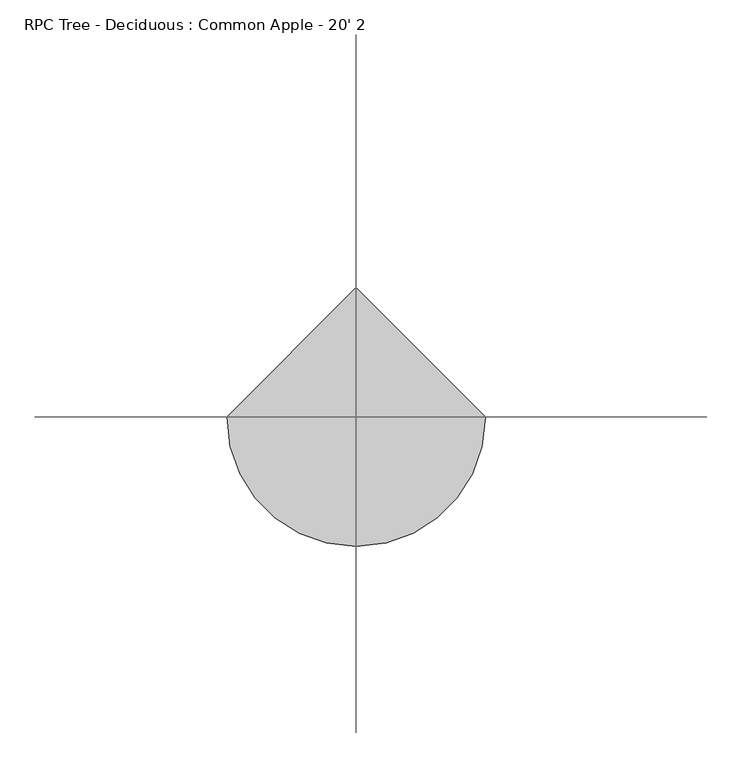
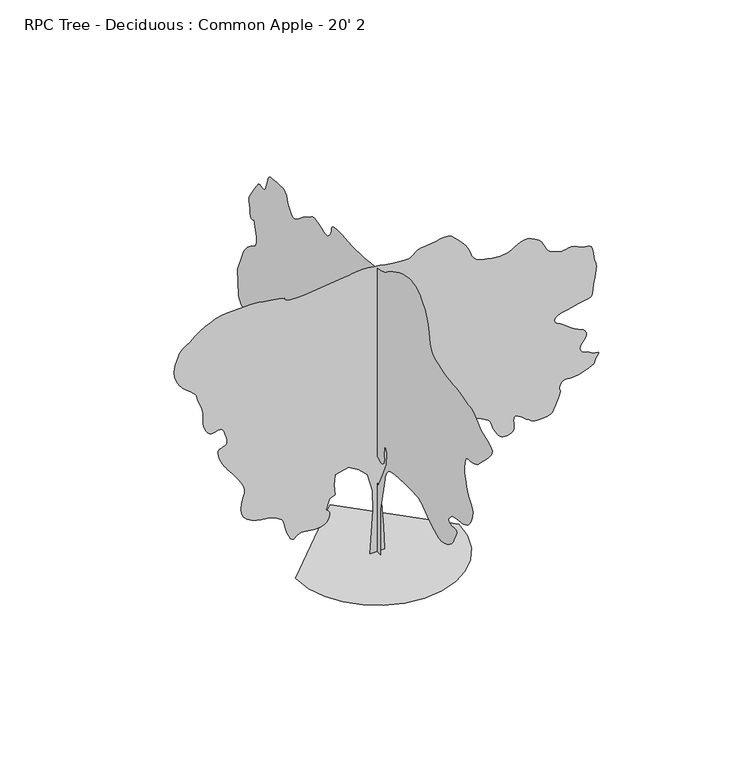
"""IFC4 building model written with IfcOpenShell, lengths in millimetres: geographic element geometry, RPC Tree - Deciduous : Common Apple - 20' 2."""

from ifc_helpers import new_model, si_unit, origin, place, context, project, spatial, triangles, source, transform, mapped, element, save


def rpc_tree_deciduous_common_apple_20_2_2cf08d23(model_context):
    return source(origin(), model_context, "Body", "Tessellation", [
        triangles([(-6.61e-05, -106.7031981, 0.0075972), (-6.25e-05, 141.1357166, 0.0075898), (-4.92e-05, 101.4814601, 465.9455781), (-3.19e-05, 131.2220957, 1031.0173004), (-1.83e-05, 230.3576144, 1437.4734501), (-8.7e-06, 398.8869896, 1675.3980263), (-1.1e-06, 587.2459139, 1834.016106), (2.7e-06, 765.6887283, 1873.6680462), (3.6e-06, 963.961219, 1804.2751888), (1.5e-06, 1023.4430534, 1705.1389435), (-4.1e-06, 904.4794573, 1576.2617809), (-8.5e-06, 944.1340136, 1407.7326782), (-1.46e-05, 1172.144878, 1090.4990622), (-1.49e-05, 1568.687534, 882.3128597), (-8.7e-06, 2143.6727863, 803.006436), (7.7e-06, 2490.6473923, 1179.7191977), (2.57e-05, 2847.5453751, 1606.0026981), (3.25e-05, 3402.6882339, 1556.4345028), (3.9e-05, 3600.9610153, 1675.3980263), (4.6e-05, 3591.0549339, 1913.3226025), (4.57e-05, 3412.6196045, 1992.6315697), (5.03e-05, 3283.7399712, 2210.7288677), (5.51e-05, 3591.0549339, 2220.6425068), (6.07e-05, 4205.6845688, 2101.6814541), (6.29e-05, 4275.3567696, 2137.8384041), (6.49e-05, 4342.3114037, 2174.2544952), (6.7e-05, 4403.9061905, 2211.1911942), (6.89e-05, 4457.4241447, 2248.9101128), (7.07e-05, 4500.1976967, 2287.6680668), (7.23e-05, 4529.5348595, 2327.7263775), (7.37e-05, 4542.7427742, 2369.3469475), (8.93e-05, 4572.4863075, 2874.9268433), (9.94e-05, 4403.9570595, 3301.215358), (0.0001002, 4386.5834106, 3334.8449913), (0.000101, 4360.9041641, 3374.6975006), (0.0001018, 4328.265168, 3418.5378479), (0.0001026, 4290.0887192, 3464.105706), (0.0001033, 4247.7471176, 3509.1651649), (0.0001039, 4202.636499, 3551.4561882), (0.0001043, 4156.1291634, 3588.718158), (0.0001045, 4111.323468, 3617.9027138), (0.0001046, 4070.8611122, 3640.1530998), (0.0001046, 4035.4281006, 3659.4571541), (0.0001048, 4005.7101471, 3679.8024239), (0.0001052, 3982.4182549, 3705.2026176), (0.000106, 3966.2384285, 3739.5941231), (0.0001073, 3957.8566727, 3786.9906487), (0.0001089, 3956.7898773, 3842.7945099), (0.0001107, 3961.4378494, 3899.6395866), (0.0001126, 3970.8614021, 3957.3738533), (0.0001145, 3984.0948967, 4015.7685448), (0.0001165, 4000.1982742, 4074.6966339), (0.0001185, 4018.2070587, 4133.9802246), (0.0001206, 4037.1553207, 4193.4417114), (0.0001203, 4062.5299347, 4172.9947037), (0.0001202, 4087.2188347, 4157.4244331), (0.0001204, 4110.5107269, 4151.5570587), (0.000121, 4131.7196068, 4160.2693176), (0.0001221, 4150.160051, 4188.3870781), (0.0001239, 4165.1460548, 4240.787368), (0.0001265, 4175.9410355, 4322.3213448), (0.000129, 4186.6092796, 4402.5600517), (0.0001308, 4198.1408432, 4455.5698975), (0.000132, 4205.3543564, 4492.9588943), (0.000133, 4202.9922913, 4526.3597626), (0.0001339, 4185.923275, 4567.406385), (0.0001352, 4148.8900703, 4627.7059021), (0.000137, 4086.736306, 4718.8666168), (0.0001389, 4019.8834099, 4816.9867905), (0.0001404, 3969.4896835, 4892.043837), (0.0001414, 3931.4405525, 4946.4759796), (0.0001421, 3901.5194138, 4982.6714447), (0.0001423, 3875.5858223, 5003.1184525), (0.0001421, 3849.5002052, 5010.2046478), (0.0001416, 3819.0709579, 5006.343837), (0.0001408, 3787.3208611, 4996.7176804), (0.0001401, 3759.4062859, 4987.6240494), (0.0001396, 3734.2601463, 4983.2045517), (0.0001394, 3710.841227, 4987.6240494), (0.0001396, 3688.1338921, 5005.0485672), (0.0001402, 3665.0704742, 5039.6435486), (0.0001416, 3640.6103394, 5095.574437), (0.0001432, 3619.2235634, 5160.9030075), (0.0001447, 3603.043737, 5219.9581238), (0.000146, 3587.5496246, 5271.4183548), (0.000147, 3568.2455704, 5313.8366959), (0.0001475, 3540.6103386, 5345.8661362), (0.0001475, 3500.1482735, 5366.109668), (0.0001469, 3442.3378487, 5373.1458664), (0.0001459, 3372.4368828, 5376.2445145), (0.0001451, 3300.6055115, 5383.3312912), (0.0001442, 3229.8412262, 5391.1034912), (0.0001434, 3163.0391991, 5396.2851517), (0.0001425, 3103.1713417, 5395.5485687), (0.0001414, 3053.2095657, 5385.642778), (0.0001402, 3016.0746231, 5363.2394943), (0.0001391, 2991.8429626, 5337.2044556), (0.0001382, 2976.4758774, 5316.3510773), (0.0001375, 2966.6462448, 5297.4283951), (0.0001368, 2959.0769394, 5277.1081238), (0.0001359, 2950.4664185, 5252.1148819), (0.0001348, 2937.5122673, 5219.1198029), (0.0001331, 2916.9382324, 5174.873085), (0.0001313, 2890.1666107, 5126.1051315), (0.0001296, 2860.6265533, 5083.2042618), (0.000128, 2827.9619774, 5048.4569641), (0.0001268, 2791.8432518, 5024.124147), (0.0001258, 2751.8890045, 5012.4399765), (0.0001253, 2707.794603, 5015.6909409), (0.0001252, 2659.1789658, 5036.0873703), (0.0001254, 2610.791803, 5068.0662323), (0.0001258, 2565.8846603, 5103.6768494), (0.0001263, 2521.8332794, 5141.7006912), (0.0001267, 2476.0523529, 5180.9436447), (0.0001272, 2425.9356445, 5220.212178), (0.0001274, 2368.8821503, 5258.2360199), (0.0001275, 2302.2908661, 5293.846637), (0.0001276, 2240.2945049, 5328.4671982), (0.0001279, 2193.5584042, 5362.0459625), (0.0001282, 2154.2798424, 5391.129071), (0.0001282, 2114.6558075, 5412.2365036), (0.0001278, 2066.8783459, 5421.8882401), (0.0001267, 2003.1496777, 5416.6304214), (0.0001247, 1915.6618492, 5392.9830276), (0.0001224, 1826.1497257, 5361.2837997), (0.0001207, 1757.9710384, 5335.9853439), (0.0001194, 1705.7434124, 5319.8816757), (0.0001187, 1664.0950825, 5315.7418121), (0.0001184, 1627.6484699, 5326.358606), (0.0001187, 1591.0293388, 5354.4766571), (0.0001195, 1548.8602558, 5402.8893997), (0.0001207, 1514.8419834, 5459.7853455), (0.000122, 1498.8602554, 5510.7630478), (0.0001232, 1489.8128426, 5554.806871), (0.0001241, 1476.6047825, 5590.874437), (0.0001244, 1448.1338459, 5617.9256927), (0.0001241, 1393.3079773, 5634.9182602), (0.0001229, 1301.0220406, 5640.8109238), (0.0001214, 1201.3955635, 5639.6935501), (0.0001202, 1126.7398006, 5636.6454803), (0.0001192, 1069.2519579, 5632.2259827), (0.0001184, 1021.1290958, 5626.9425842), (0.0001175, 974.5682751, 5621.3039749), (0.0001165, 921.7642307, 5615.8426804), (0.0001154, 854.9113346, 5611.0679718), (0.0001143, 784.7082069, 5608.019902), (0.0001133, 723.0014357, 5607.2071609), (0.0001125, 663.7228592, 5608.4768509), (0.0001116, 600.8019178, 5611.6516571), (0.0001107, 528.1680156, 5616.5792633), (0.0001096, 439.7556433, 5623.0567749), (0.0001082, 329.4941322, 5630.9051331), (0.0001067, 206.9466705, 5641.7254028), (0.0001053, 88.3885184, 5656.6861176), (0.0001042, -22.1921751, 5675.1262711), (0.0001034, -120.8075788, 5696.3354416), (0.0001029, -203.4686488, 5719.6276245), (0.0001027, -266.1871316, 5744.3162338), (0.0001028, -304.9729546, 5769.6908478), (0.0001032, -347.9523442, 5804.4381454), (0.0001036, -420.583703, 5853.4089935), (0.0001039, -514.8939712, 5910.1532043), (0.000104, -622.9024584, 5968.31884), (0.0001039, -736.6335978, 6021.4301331), (0.0001035, -848.1092062, 6063.1118912), (0.0001027, -949.3562239, 6086.9371811), (0.0001016, -1039.2697763, 6095.8017563), (0.0001004, -1122.4243664, 6096.0046509), (9.9e-05, -1199.3330441, 6086.1494385), (9.73e-05, -1270.5191059, 6064.8391113), (9.53e-05, -1336.5033051, 6030.7016602), (9.29e-05, -1397.8062492, 5982.3650757), (9.01e-05, -1454.9462208, 5918.407933), (8.77e-05, -1502.3755932, 5861.1056168), (8.62e-05, -1536.9730453, 5825.4944183), (8.5e-05, -1562.8963177, 5799.256485), (8.38e-05, -1584.313615, 5770.0716385), (8.22e-05, -1605.3828232, 5725.6220261), (7.96e-05, -1630.2698215, 5653.5874695), (7.58e-05, -1663.1323505, 5541.6751144), (7.16e-05, -1693.8258259, 5415.6147858), (6.81e-05, -1715.6747829, 5307.5626602), (6.5e-05, -1738.0446384, 5214.9799393), (6.21e-05, -1770.3000824, 5135.1981812), (5.93e-05, -1821.8062408, 5065.6530075), (5.62e-05, -1901.9230076, 5003.7532974), (5.28e-05, -2020.0178341, 4946.8823502), (4.95e-05, -2152.913356, 4902.7117905), (4.69e-05, -2273.494804, 4876.3974083), (4.48e-05, -2385.2295536, 4861.5384315), (4.29e-05, -2491.5921021, 4851.7340881), (4.1e-05, -2596.0345642, 4840.5071571), (3.89e-05, -2702.0542557, 4821.482737), (3.62e-05, -2813.1030006, 4788.2594742), (3.39e-05, -2912.3155495, 4758.5159409), (3.24e-05, -2986.585144, 4746.9843773), (3.14e-05, -3044.8780975, 4742.742485), (3.04e-05, -3096.2371719, 4734.8432579), (2.89e-05, -3149.6786774, 4712.3896866), (2.66e-05, -3214.2200867, 4664.4344742), (2.28e-05, -3298.878582, 4580.0809021), (1.85e-05, -3408.6320572, 4492.8062874), (1.5e-05, -3530.0185432, 4434.3354378), (1.2e-05, -3644.3188339, 4390.95233), (9.4e-06, -3732.7616913, 4348.9659393), (7.2e-06, -3776.6273277, 4294.6608238), (5.1e-06, -3757.196537, 4214.3459587), (3e-06, -3655.7486595, 4094.3056114), (1.1e-06, -3529.027906, 3968.7786804), (-3e-07, -3439.3912262, 3876.7287758), (-1.3e-06, -3376.6531952, 3811.5525215), (-1.9e-06, -3330.5522301, 3766.670668), (-2.3e-06, -3290.852037, 3735.479258), (-2.3e-06, -3247.3671913, 3711.4002045), (-2.2e-06, -3189.8108208, 3687.854258), (-1.7e-06, -3124.3802216, 3671.1919029), (-1e-06, -3064.487075, 3666.3404549), (-2e-07, -3010.8420937, 3664.4356293), (2e-07, -2964.1568619, 3656.6378494), (2e-07, -2925.0662247, 3634.0825401), (-8e-07, -2894.3070557, 3587.9559952), (-2.8e-06, -2872.5897766, 3509.3939301), (-5.1e-06, -2860.8041588, 3423.8465355), (-7.1e-06, -2858.3659355, 3357.9081184), (-8.8e-06, -2863.7507813, 3304.4410332), (-1.04e-05, -2875.358503, 3256.3335045), (-1.21e-05, -2891.6653564, 3206.498465), (-1.41e-05, -2911.070858, 3147.8244301), (-1.67e-05, -2932.0768433, 3073.199334), (-1.95e-05, -2961.2613991, 2993.8242371), (-2.22e-05, -3001.7234642, 2923.6186386), (-2.47e-05, -3046.5291595, 2859.6612053), (-2.72e-05, -3088.7187355, 2798.9806068), (-2.95e-05, -3121.3830208, 2738.6555099), (-3.16e-05, -3137.5628471, 2675.7398735), (-3.35e-05, -3130.349334, 2607.2612045), (-3.52e-05, -3109.3942177, 2540.281572), (-3.66e-05, -3087.7280983, 2482.819091), (-3.77e-05, -3063.4964378, 2433.5098915), (-3.85e-05, -3034.7182526, 2390.964814), (-3.91e-05, -2999.5645844, 2353.7970245), (-3.94e-05, -2956.0544495, 2320.6169277), (-3.96e-05, -2902.3333099, 2290.0378349), (-3.93e-05, -2836.3948929, 2266.2507694), (-3.86e-05, -2760.9314758, 2251.4832115), (-3.77e-05, -2680.9721123, 2241.3942924), (-3.68e-05, -2601.4955681, 2231.6559334), (-3.61e-05, -2527.6041481, 2217.9272655), (-3.58e-05, -2464.279525, 2195.8749779), (-3.62e-05, -2416.56049, 2161.1632885), (-3.68e-05, -2383.2356346, 2123.2410393), (-3.73e-05, -2359.9691769, 2093.2995529), (-3.79e-05, -2347.1065899, 2069.598674), (-3.84e-05, -2344.9984337, 2050.4090023), (-3.9e-05, -2353.9875652, 2033.9929985), (-3.98e-05, -2374.4217831, 2018.6158848), (-4.07e-05, -2406.646851, 2002.5452087), (-4.16e-05, -2449.8269188, 1993.9041664), (-4.23e-05, -2498.3841293, 1996.5330757), (-4.28e-05, -2545.5646797, 2002.2862129), (-4.34e-05, -2584.5791588, 2003.0075352), (-4.41e-05, -2608.6837921, 1990.5513187), (-4.52e-05, -2611.0967262, 1956.7642822), (-4.66e-05, -2585.0869766, 1893.4953243), (-4.83e-05, -2549.9080193, 1821.1814243), (-4.96e-05, -2524.6272949, 1762.91376), (-5.07e-05, -2502.1126808, 1714.5318295), (-5.16e-05, -2475.2625755, 1671.8725147), (-5.23e-05, -2436.9668026, 1630.7726978), (-5.27e-05, -2380.1140228, 1587.0720222), (-5.3e-05, -2297.5969666, 1536.6072247), (-5.28e-05, -2203.8378639, 1496.8968578), (-5.19e-05, -2116.842738, 1484.7582092), (-5.03e-05, -2034.8743401, 1494.9892708), (-4.83e-05, -1956.2028339, 1522.3883251), (-4.6e-05, -1879.090971, 1561.7532188), (-4.35e-05, -1801.803828, 1607.8822346), (-4.09e-05, -1722.6115688, 1655.5707481), (-3.83e-05, -1647.9584221, 1703.6352562), (-3.59e-05, -1583.013113, 1752.3931812), (-3.37e-05, -1524.1383636, 1798.8980461), (-3.16e-05, -1467.6919544, 1840.2010483), (-2.97e-05, -1410.0313751, 1873.3506237), (-2.82e-05, -1347.5167316, 1895.4053822), (-2.69e-05, -1276.503479, 1903.4089634), (-2.54e-05, -1177.6846561, 1904.2776604), (-2.33e-05, -1044.3574018, 1905.4916851), (-2.11e-05, -891.7820492, 1904.9710773), (-1.89e-05, -735.2163151, 1900.6352955), (-1.7e-05, -589.9230761, 1890.4040886), (-1.58e-05, -471.1627742, 1872.1948803), (-1.55e-05, -394.1956335, 1843.9297451), (-1.6e-05, -348.7041879, 1805.3140789), (-1.68e-05, -313.0958962, 1758.377409), (-1.8e-05, -285.7248199, 1704.5039532), (-1.95e-05, -264.9450744, 1645.0805454), (-2.11e-05, -249.1058704, 1581.494165), (-2.29e-05, -236.5620685, 1515.1341167), (-2.48e-05, -225.6659676, 1447.3870892), (-3.91e-05, -116.6168281, 912.0537769), (-2.05e-05, -27.3946828, 1318.5099266), (-1.32e-05, -176.0980811, 1635.74347), (-6.6e-06, -304.975498, 1923.2362415), (2e-07, -324.8002327, 2161.1632885), (4.8e-06, -255.4073572, 2280.1241959), (-4e-07, -225.6657133, 2091.767815), (-1.7e-06, -231.7353101, 2049.4539734), (-3e-06, -235.984215, 2008.1814926), (-4.2e-06, -236.5910275, 1968.9892628), (-5.2e-06, -231.7353101, 1932.9186447), (-6e-06, -219.5961346, 1901.0111446), (-6.5e-06, -198.3530817, 1874.3056526), (-6.6e-06, -166.1844602, 1853.8433842), (-6.2e-06, -129.2182845, 1848.5829494), (-5.3e-06, -95.0268123, 1860.3152275), (-4.3e-06, -63.9562343, 1879.3348515), (-3.4e-06, -36.354542, 1895.9235191), (-2.9e-06, -12.5678035, 1900.3761543), (-3.1e-06, 7.0569383, 1882.9772163), (-4.4e-06, 22.1729471, 1834.016106), (-6.1e-06, 32.8958209, 1768.9260384), (-7.8e-06, 39.9768386, 1709.0403042), (-9.4e-06, 44.0233167, 1653.4904972), (-1.1e-05, 45.6418044, 1601.4077751), (-1.24e-05, 45.4396183, 1551.9260571), (-1.39e-05, 44.0233167, 1504.1789715), (-1.53e-05, 41.9999482, 1457.3007282), (139.590126, 0.0003305, 0.0), (-135.4471285, 0.0003387, 0.0), (-74.3278259, 0.000241, 845.4879272), (-84.5142454, 0.0002472, 1242.76455), (-186.3807747, 0.0002013, 1599.294532), (-339.1791879, 0.0002082, 1752.0933449), (-542.9102117, 0.000216, 1874.3335579), (-797.5758808, 0.0002227, 1813.2134514), (-817.9492012, 0.0002203, 1609.4824276), (-797.5758808, 0.0002168, 1415.9368286), (-899.4426281, 0.0002191, 1365.0021469), (-970.7481594, 0.0002183, 1171.4565479), (-951.3247084, 0.0002718, 1158.1240768), (-933.2373676, 0.000271, 1143.3616058), (-917.8246456, 0.0002703, 1125.7517796), (-906.4200365, 0.0002696, 1103.8645981), (-900.3621214, 0.000269, 1076.2750757), (-900.9870106, 0.0002686, 1041.555756), (-909.6280529, 0.0002682, 998.2868128), (-928.5764603, 0.0002681, 955.1042742), (-957.6798437, 0.0002684, 921.0098436), (-994.6267164, 0.0002692, 895.1144766), (-1037.0955631, 0.0002701, 876.5217161), (-1082.7698101, 0.0002713, 864.3449158), (-1129.3382612, 0.0002726, 857.6926329), (-1174.4791832, 0.0002739, 855.6733521), (-1218.6700905, 0.0002753, 858.4063974), (-1263.5747623, 0.0002767, 865.0586803), (-1308.6573303, 0.0002782, 873.3161705), (-1353.3816353, 0.0002796, 880.857498), (-1397.217041, 0.000281, 885.3710306), (-1439.6273884, 0.0002823, 884.5404854), (-1480.0769543, 0.0002833, 876.0466724), (-1514.854628, 0.0002841, 857.900905), (-1542.5051205, 0.0002846, 834.4084436), (-1565.8782578, 0.000285, 812.6990856), (-1587.8238659, 0.0002854, 799.9000122), (-1611.1970032, 0.0002862, 803.1359339), (-1638.8473503, 0.0002874, 829.5392641), (-1673.6225533, 0.000235, 886.2346407), (-1706.6171963, 0.0002371, 959.4984827), (-1729.2790398, 0.0002388, 1029.5593225), (-1744.988982, 0.0002402, 1094.4487484), (-1757.1353336, 0.0002415, 1152.2135365), (-1769.1037891, 0.0002426, 1200.8900711), (-1784.2803337, 0.0002436, 1238.5177162), (-1806.0481911, 0.0002446, 1263.1378704), (-1833.1626698, 0.0002457, 1282.7670502), (-1863.3073414, 0.0002469, 1305.4288937), (-1898.2629112, 0.0002483, 1329.1576778), (-1939.8122646, 0.0002499, 1351.9948013), (-1989.7334908, 0.0002517, 1371.9820988), (-2049.8147072, 0.0002537, 1387.1586433), (-2121.8338577, 0.000256, 1395.5635082), (-2205.4938675, 0.0002044, 1404.6210949), (-2294.67854, 0.0002073, 1424.3695988), (-2382.4381542, 0.0002104, 1456.7724174), (-2461.8232796, 0.0002135, 1503.7853909), (-2525.8821602, 0.0002163, 1567.3691551), (-2567.6627495, 0.0002188, 1649.4849277), (-2580.2355286, 0.0002207, 1752.0933449), (-2568.9835991, 0.0002218, 1851.4048702), (-2548.8159348, 0.0002224, 1927.9097935), (-2527.0379036, 0.0002227, 1989.979842), (-2510.9723145, 0.0001688, 2045.9893593), (-2507.9117455, 0.0001695, 2104.3180664), (-2525.1659248, 0.0001711, 2173.3375454), (-2570.0503944, 0.0001737, 2261.4222851), (-2629.7912247, 0.0001769, 2355.7756828), (-2686.3316689, 0.0001798, 2438.7243988), (-2738.9604332, 0.0001825, 2511.3356644), (-2786.9665146, 0.0001849, 2574.6730774), (-2829.6130394, 0.0001327, 2629.841803), (-2866.1890045, 0.0001345, 2677.8478844), (-2896.008696, 0.000136, 2719.8086952), (-2924.6092758, 0.0001376, 2767.4084061), (-2955.1652596, 0.0001394, 2827.2762634), (-2983.4100471, 0.0001412, 2893.0114952), (-3005.0764572, 0.0001428, 2958.2389091), (-3015.8461487, 0.000144, 3016.5062828), (-3011.4772293, 0.0001446, 3061.4137161), (-2987.7028084, 0.0001442, 3086.5342758), (-2951.4823448, 0.0001433, 3098.8532913), (-2915.109565, 0.0001425, 3111.5533882), (-2882.1147766, 0.0001417, 3127.4282913), (-2856.0800285, 0.0001413, 3149.3740448), (-2840.5350471, 0.0001413, 3180.2349518), (-2839.0871704, 0.0001418, 3222.8561874), (-2855.2669968, 0.0001432, 3280.0823456), (-2877.0348541, 9.05e-05, 3338.9342766), (-2892.2240433, 9.16e-05, 3385.5177704), (-2904.1875572, 9.25e-05, 3421.2048363), (-2916.3286766, 9.32e-05, 3447.4686401), (-2932.0259743, 9.4e-05, 3465.705899), (-2954.70802, 9.48e-05, 3477.3389099), (-2987.7028084, 9.59e-05, 3483.8161308), (-3026.4123642, 9.7e-05, 3481.8857254), (-3064.2583099, 9.8e-05, 3472.1066711), (-3101.5455688, 9.9e-05, 3461.6419029), (-3138.6805115, 0.0001, 3457.552327), (-3175.9930595, 0.0001013, 3467.026458), (-3213.8137161, 0.0001029, 3497.1763618), (-3252.5488518, 0.0001049, 3555.1138138), (-3281.1747208, 0.0001068, 3626.7419998), (-3293.239682, 0.0001082, 3695.3474052), (-3295.8558014, 0.0001093, 3764.1307068), (-3296.1351448, 0.0001104, 3836.3175797), (-3301.2406471, 5.74e-05, 3915.0575409), (-3318.2840836, 5.93e-05, 4003.6274254), (-3354.4028091, 6.19e-05, 4105.2020393), (-3391.2836975, 6.43e-05, 4197.0231789), (-3411.2481766, 6.59e-05, 4259.8120789), (-3422.2972115, 6.68e-05, 4301.925206), (-3432.4570564, 6.76e-05, 4331.7448975), (-3449.7545471, 6.85e-05, 4357.6276199), (-3482.1650688, 6.99e-05, 4387.9804184), (-3537.7657448, 7.22e-05, 4431.1606316), (-3609.6985634, 2.09e-05, 4488.5646858), (-3681.631382, 2.41e-05, 4556.1285851), (-3747.3157448, 2.72e-05, 4634.0305161), (-3800.5287758, 3.01e-05, 4722.4480843), (-3835.047599, 3.26e-05, 4821.5588951), (-3844.6231773, 3.45e-05, 4931.5152649), (-3822.9823471, 3.57e-05, 5052.5468307), (-3789.555899, -1.8e-05, 5157.9310959), (-3763.7749146, -1.77e-05, 5228.187854), (-3739.5941231, -1.77e-05, 5274.3902664), (-3710.9682541, -1.81e-05, 5307.5882401), (-3671.8270386, -1.88e-05, 5338.8555176), (-3616.1246246, -1.98e-05, 5379.1652664), (-3537.7657448, -2.13e-05, 5439.6429703), (-3445.4364967, -2.3e-05, 5511.6775269), (-3351.6849518, -2.48e-05, 5578.225209), (-3256.3079247, -2.67e-05, 5637.4326416), (-3159.1783882, -2.89e-05, 5687.5726044), (-3060.0675774, -3.12e-05, 5726.8155579), (-2958.8228851, -3.39e-05, 5753.4348633), (-2855.2669968, -3.68e-05, 5765.6015625), (-2376.4970924, -5.09e-05, 5775.7869873), (-2309.7356152, -5.29e-05, 5773.1197083), (-2232.8167637, -5.53e-05, 5765.6521408), (-2147.4320045, -3.8e-06, 5754.1458664), (-2055.2781818, -6.7e-06, 5739.4392059), (-1958.0469074, -9.9e-06, 5722.3449005), (-1857.4273224, -1.32e-05, 5703.6251129), (-1755.1159801, -1.65e-05, 5684.1181641), (-1751.9080364, -1.69e-05, 5664.6617935), (-1742.5530842, -1.75e-05, 5646.3739563), (-1720.9022255, -1.83e-05, 5630.3970245), (-1680.8107773, -1.97e-05, 5617.9001129), (-1616.1270802, -2.18e-05, 5610.0261749), (-1520.7042709, -2.46e-05, 5607.9437439), (-1388.3981026, -2.85e-05, 5612.8201904), (-614.2181774, -5.02e-05, 5704.4890137), (-538.3076946, -5.24e-05, 5711.4996323), (-472.1990845, 1e-07, 5721.8879517), (-409.4762778, -1.6e-06, 5732.8355392), (-343.7232419, -3.5e-06, 5741.4460602), (-268.5264692, -5.7e-06, 5744.8749207), (-177.4707081, -8.5e-06, 5740.3031067), (-64.1414019, -1.21e-05, 5724.8598633), (54.7118994, -1.59e-05, 5704.3111176), (159.4882483, -1.93e-05, 5686.4296509), (252.3260954, -2.23e-05, 5671.4183578), (335.3640864, -2.49e-05, 5659.4039749), (410.7386644, -2.73e-05, 5650.6155579), (480.5886887, -2.95e-05, 5645.205423), (547.0529457, -3.15e-05, 5643.3764648), (603.2428662, -3.3e-05, 5651.8346695), (646.0698669, -3.4e-05, 5673.6531052), (683.3697704, -3.47e-05, 5703.4983765), (722.9887184, -3.54e-05, 5736.0359253), (772.7625698, -3.64e-05, 5765.8806152), (840.5349592, -3.81e-05, 5787.6996323), (934.1441437, -4.07e-05, 5796.1828354), (1035.6832947, -4.37e-05, 5802.989978), (1124.0372766, -4.61e-05, 5818.3826431), (1202.2337391, -4.82e-05, 5834.6642075), (1273.3004768, -5.01e-05, 5844.1636276), (1340.2726971, -5.22e-05, 5839.2360214), (1406.173035, -5.46e-05, 5812.2103455), (1474.0342999, -3.2e-06, 5755.4161377), (1539.0152172, -6.2e-06, 5686.9627579), (1594.7301304, -8.7e-06, 5628.1366974), (1641.8903332, -1.09e-05, 5576.0666199), (1681.2120609, -1.28e-05, 5527.9335114), (1713.4041367, -1.44e-05, 5480.8671982), (1739.182505, -1.59e-05, 5431.9975067), (1759.2587505, -1.73e-05, 5378.5304214), (1777.3156425, -1.87e-05, 5324.8604416), (1798.9361252, -2e-05, 5277.2604401), (1827.6839344, -2.15e-05, 5235.5281036), (1867.1225155, 3.1e-05, 5199.4855362), (1920.8180752, 2.9e-05, 5169.0060013), (1992.3318787, 2.65e-05, 5143.8342819), (2085.229842, 2.34e-05, 5123.844223), (2181.6306438, 2.03e-05, 5109.4171967), (2262.7075264, 1.78e-05, 5100.6799393), (2330.5991673, 1.57e-05, 5097.123761), (2387.4419186, 1.4e-05, 5098.1905563), (2435.3767834, 1.27e-05, 5103.3722168), (2476.5374977, 1.16e-05, 5112.0844757), (2513.0678261, 1.07e-05, 5123.844223), (2552.2195061, 9.8e-06, 5144.4947067), (2599.1840813, 8.9e-06, 5175.4829315), (2653.1336952, 7.8e-06, 5209.6459625), (2713.1032906, 6.4e-06, 5239.9226028), (2778.2795448, 4.8e-06, 5259.1249191), (2847.697982, 2.7e-06, 5260.1661346), (2920.5196999, 2e-07, 5235.9094757), (2984.2992371, -2.2e-06, 5202.1528152), (3030.2478859, -4e-06, 5176.5747253), (3062.9883293, -5.3e-06, 5154.908606), (3087.1947006, -6.3e-06, 5132.9122742), (3107.4893921, -7.3e-06, 5106.2679703), (3128.4697975, -8.5e-06, 5070.73293), (3154.8094688, -1e-05, 5021.9905563), (3182.8510712, 4.27e-05, 4971.0890121), (3208.2256851, 4.13e-05, 4930.3473129), (3234.4639091, 4e-05, 4897.4289734), (3265.1724998, 3.87e-05, 4870.0475052), (3303.9076355, 3.72e-05, 4845.8667137), (3354.2252037, 3.53e-05, 4822.6004013), (3419.6808014, 3.3e-05, 4797.8859215), (3486.0258797, 3.08e-05, 4782.8237595), (3540.0769409, 2.92e-05, 4784.7032959), (3586.9909378, 2.8e-05, 4795.4729874), (3631.9489494, 2.68e-05, 4807.1571579), (3680.1326363, 2.55e-05, 4811.7036827), (3736.6730804, 2.36e-05, 4801.0863075), (3806.7519424, 2.1e-05, 4767.3299377), (3879.2181587, 1.84e-05, 4732.9890106), (3939.9240463, 1.63e-05, 4718.4346664), (3989.5811897, 1.48e-05, 4712.2626595), (4028.9003014, 1.35e-05, 4703.0678719), (4058.6185455, 1.22e-05, 4679.4204781), (4079.3957657, 6.51e-05, 4629.9412308), (4091.9941246, 6.34e-05, 4543.2253029), (4103.8306114, 6.18e-05, 4454.6301292), (4119.4261711, 6.04e-05, 4397.0481789), (4135.0217308, 5.94e-05, 4355.3161331), (4146.8835068, 5.84e-05, 4314.2950905), (4151.2268463, 5.74e-05, 4258.8467308), (4144.3688347, 5.64e-05, 4173.8330246), (4122.550399, 5.51e-05, 4044.0642014), (4100.096537, 0.000108, 3908.7329269), (4088.8698967, 0.0001069, 3812.0603394), (4081.3767494, 0.0001061, 3746.5791618), (4070.1501091, 0.0001058, 3704.7962471), (4047.6965378, 0.0001061, 3679.2184479), (4006.548468, 0.0001071, 3662.4034859), (3939.1874634, 0.0001089, 3646.8079262), (3844.4708611, 0.0001114, 3628.5706673), (3734.0822502, 0.0001144, 3608.1998177), (3619.7822502, 0.0001175, 3584.781189), (3513.3053192, 0.0001202, 3557.4761696), (3426.4373657, 0.0001224, 3525.3449913), (3370.9384277, 0.0001234, 3487.4990456), (3358.5429634, 0.0001231, 3443.0744316), (3371.5224037, 0.0001222, 3405.6092766), (3386.2799332, 0.0001214, 3384.1972115), (3405.8633308, 0.0001207, 3371.1669022), (3433.2700882, 0.0001197, 3358.8478867), (3471.5476936, 0.0001182, 3339.5694122), (3523.7447983, 0.0001162, 3305.6857246), (3592.8327324, 0.0001133, 3249.5260712), (3669.2870773, 0.0001101, 3189.9884262), (3740.381575, 0.0001074, 3147.3671906), (3804.5419029, 0.000105, 3116.150782), (3860.1425789, 0.0001572, 3090.8014572), (3905.55783, 0.0001555, 3065.8332138), (3939.2383324, 0.000154, 3035.6833099), (3959.558313, 0.0001528, 2994.8654526), (3960.2948959, 0.0001521, 2946.884951), (3941.8038734, 0.0001519, 2899.2852402), (3912.2635254, 0.0001521, 2852.3968231), (3879.8530037, 0.0001524, 2806.5752014), (3852.8020386, 0.0001525, 2762.1758766), (3839.2892006, 0.0001523, 2719.554641), (3847.5189308, 0.0001514, 2679.0672867), (3870.582058, 0.0001503, 2647.1645828), (3896.1598572, 0.0001492, 2627.2256836), (3924.2270393, 0.0001482, 2614.9319572), (3954.7830231, 0.0001472, 2606.0168037), (3987.8286804, 0.000146, 2596.2121696), (4023.3887192, 0.0001447, 2581.2517456), (4061.4378502, 0.0001432, 2556.842189), (4100.7569618, 0.0001417, 2534.5891869), (4137.7648773, 0.0001405, 2524.8203064), (4168.8798386, 0.0001395, 2521.2847664), (4190.5462486, 0.0001388, 2517.7515518), (4199.2329277, 0.0001384, 2507.9803459), (4191.3334099, 0.0001926, 2485.7375175), (4163.2918076, 0.0001928, 2444.7824593), (4135.3263634, 0.0001929, 2399.7888393), (4122.8550316, 0.0001928, 2366.7332989), (4115.1842789, 0.0001927, 2341.3408081), (4101.6461517, 0.0001927, 2319.3343025), (4071.521537, 0.0001933, 2296.4387524), (4014.1430626, 0.0001946, 2268.3717155), (3918.8166138, 0.0001969, 2230.8633945), (3811.1205711, 0.0001996, 2200.6297749), (3722.1443161, 0.0002021, 2191.0666958), (3649.3987564, 0.0002043, 2192.9081532), (3590.3436401, 0.0002062, 2196.8884335), (3542.540744, 0.0002075, 2193.7413872), (3503.4501068, 0.0002084, 2174.1985394), (3470.6079254, 0.0002087, 2128.9966473), (3451.2532928, 0.0002086, 2081.7474964), (3449.1702805, 0.0002083, 2055.3443115), (3456.7142967, 0.0002078, 2039.4564732), (3466.2137169, 0.0002073, 2023.7466763), (3470.0236588, 0.0002068, 1997.8792145), (3460.4480804, 0.0002064, 1951.5191082), (3429.8662262, 0.0002061, 1874.3335579), (3393.2393921, 0.0002059, 1787.376511), (3366.4171921, 0.0002057, 1717.5239433), (3342.9982727, 0.0002056, 1663.1755165), (3316.5315742, 0.0002058, 1622.7259506), (3280.6157433, 0.0002064, 1594.5725819), (3228.850589, 0.0002077, 1577.1101303), (3154.8094688, 0.0002098, 1568.7357868), (3080.6413216, 0.0002119, 1565.2609989), (3027.8349518, 0.0002135, 1564.6361824), (2989.0998161, 0.0002147, 1568.469088), (2957.146534, 0.0002158, 1578.3572926), (2924.6598541, 0.000217, 1595.9086922), (2884.3248161, 0.0002186, 1622.7259506), (2828.8511673, 0.0002209, 1660.4146385), (2768.830703, 0.0002233, 1702.4363468), (2719.1482704, 0.0002253, 1739.6499184), (2678.9146797, 0.000227, 1769.7336926), (2647.2154518, 0.0002282, 1790.3763279), (2623.1869766, 0.0002291, 1799.2561638), (2605.9403549, 0.0002295, 1794.0567719), (2594.5613983, 0.0002295, 1772.4668106), (2588.1350464, 0.0002293, 1744.7273701), (2585.6459541, 0.000229, 1721.445797), (2586.0014557, 0.0002287, 1700.833683), (2588.1350464, 0.0002283, 1681.1130844), (2591.00522, 0.0002279, 1660.5034412), (2593.494603, 0.0002275, 1637.219252), (2594.5613983, 0.0002271, 1609.4824276), (2593.1135216, 0.0002267, 1579.0989624), (2587.906572, 0.0002264, 1549.7873795), (2577.7211472, 0.0002263, 1522.6143288), (2561.2872665, 0.0002264, 1498.6468964), (2537.3884346, 0.0002268, 1478.9568192), (2504.7494385, 0.0002276, 1464.6108925), (2462.1331444, 0.0002288, 1456.6836147), (2418.7144283, 0.00023, 1454.9893867), (2382.9562912, 0.0002312, 1459.35569), (2352.5447754, 0.0002322, 1470.8491745), (2325.1635979, 0.0002333, 1490.5392517), (2298.4935688, 0.0002346, 1519.4951878), (2270.2207306, 0.000236, 1558.7865395), (2238.0288002, 0.0002377, 1609.4824276), (2208.2396301, 0.0002394, 1664.8392231), (2186.8274197, 0.0001866, 1716.8127949), (2170.9397266, 0.0001878, 1764.5088661), (2157.7241089, 0.0001888, 1807.0362122), (2144.3307404, 0.0001897, 1843.5054977), (2127.9070335, 0.0001907, 1873.0254982), (2105.6033077, 0.0001917, 1894.7068783), (2074.6583942, 0.0001929, 1913.6528149), (2035.1589157, 0.0001944, 1935.2732975), (1988.5319653, 0.0001961, 1959.1214058), (1936.2028919, 0.0001981, 1984.7525448), (1879.5964634, 0.0002001, 2011.717178), (1820.1400635, 0.0002023, 2039.5759426), (1759.2587505, 0.0002046, 2067.8791569), (1412.9141933, 0.0002149, 2067.8791569), (1219.3685944, 0.0002173, 1843.7721966), (1214.8270838, 0.000217, 1813.2134514), (1209.2136909, 0.0002167, 1782.6522354), (1201.4616205, 0.0002165, 1752.0933449), (1190.5040045, 0.0002164, 1721.5345997), (1175.2665625, 0.0002164, 1690.9733837), (1154.6874407, 0.0002165, 1660.4146385), (1127.6898153, 0.0002169, 1629.855748), (1103.6638836, 0.0002172, 1604.0163368), (1088.903956, 0.0002174, 1586.5538853), (1077.7076191, 0.0002175, 1575.8629681), (1064.3726046, 0.0002179, 1570.3384506), (1043.1966442, 0.0002185, 1568.3775238), (1008.4798679, 0.0002195, 1568.3775238), (954.5175367, 0.0002211, 1568.7357868), (886.9839409, 0.0002232, 1571.6161343), (817.1339167, 0.0002254, 1579.3072346), (747.6394667, 0.0002276, 1590.3841747), (681.1726662, 0.0002298, 1603.4220417), (620.41075, 0.0002318, 1616.9957771), (568.0206702, 0.0002335, 1629.6755264), (526.6821324, 0.0002349, 1640.0411728), (491.1627162, 0.0002361, 1650.5543392), (454.5739975, 0.0002374, 1664.275304), (417.0937271, 0.0002388, 1680.6684895), (378.9022719, 0.0002402, 1699.2003525), (340.1748393, 0.0001874, 1719.3350246), (301.0918324, 0.0001889, 1740.5414337), (261.828495, 0.0001904, 1762.2813858), (78.4708189, 0.0002443, 1375.1901878), (68.2843994, 0.0002402, 1079.7776962), (119.217278, 0.0002837, 458.3966929), (-1547.0796959, 1.1e-06, 0.0099807), (-1506.1805935, -354.4877738, 0.0099913), (-1389.6986046, -680.02964, 0.010001), (-1206.9607035, -967.2962626, 0.0100095), (-967.2962626, -1206.9607035, 0.0100167), (-680.02964, -1389.6986046, 0.0100221), (-354.4877738, -1506.1805935, 0.0100256), (6.76e-05, -1547.0796959, 0.0100268), (354.4877738, -1506.1805935, 0.0100256), (680.02964, -1389.6986046, 0.0100221), (967.2962626, -1206.9607035, 0.0100167), (1206.9607035, -967.2962626, 0.0100095), (1389.6986046, -680.02964, 0.010001), (1506.1805935, -354.4877738, 0.0099913), (1547.0796959, 0.0001258, 0.0099807), (-0.0002029, 1547.0796959, 0.0099346)], [[300, 1, 301], [299, 300, 301], [299, 301, 302], [298, 299, 302], [297, 298, 302], [296, 297, 302], [296, 302, 303], [295, 296, 303], [294, 295, 303], [293, 294, 303], [292, 293, 303], [1, 2, 3], [301, 1, 3], [301, 3, 4], [301, 4, 5], [327, 301, 5], [326, 327, 5], [326, 5, 6], [325, 326, 6], [324, 325, 6], [323, 324, 6], [322, 323, 6], [321, 322, 6], [320, 321, 6], [19, 20, 21], [18, 19, 21], [17, 18, 21], [17, 21, 22], [320, 6, 7], [319, 320, 7], [291, 292, 303], [291, 303, 304], [290, 291, 304], [261, 262, 263], [260, 261, 263], [260, 263, 264], [259, 260, 264], [259, 264, 265], [258, 259, 265], [10, 11, 12], [14, 15, 16], [258, 265, 266], [257, 258, 266], [205, 206, 207], [204, 205, 207], [204, 207, 208], [203, 204, 208], [203, 208, 209], [202, 203, 209], [202, 209, 210], [257, 266, 267], [10, 12, 13], [257, 267, 268], [257, 268, 269], [256, 257, 269], [256, 269, 270], [256, 270, 271], [255, 256, 271], [255, 271, 272], [255, 272, 273], [255, 273, 274], [255, 274, 275], [255, 275, 276], [255, 276, 277], [254, 255, 277], [254, 277, 278], [254, 278, 279], [254, 279, 280], [253, 254, 280], [253, 280, 281], [253, 281, 282], [289, 290, 304], [10, 13, 14], [10, 14, 16], [10, 16, 17], [10, 17, 22], [9, 10, 22], [201, 202, 210], [201, 210, 211], [201, 211, 212], [201, 212, 213], [201, 213, 214], [201, 214, 215], [201, 215, 216], [201, 216, 217], [201, 217, 218], [201, 218, 219], [200, 201, 219], [199, 200, 219], [198, 199, 219], [197, 198, 219], [196, 197, 219], [195, 196, 219], [194, 195, 219], [194, 219, 220], [193, 194, 220], [192, 193, 220], [191, 192, 220], [190, 191, 220], [189, 190, 220], [189, 220, 221], [188, 189, 221], [252, 253, 282], [252, 282, 283], [188, 221, 222], [187, 188, 222], [251, 252, 283], [187, 222, 223], [23, 24, 25], [318, 319, 7], [56, 57, 58], [56, 58, 59], [55, 56, 59], [55, 59, 60], [54, 55, 60], [54, 60, 61], [54, 61, 62], [23, 25, 26], [186, 187, 223], [23, 26, 27], [23, 27, 28], [23, 28, 29], [23, 29, 30], [23, 30, 31], [23, 31, 32], [23, 32, 33], [23, 33, 34], [23, 34, 35], [23, 35, 36], [23, 36, 37], [23, 37, 38], [23, 38, 39], [23, 39, 40], [23, 40, 41], [23, 41, 42], [23, 42, 43], [23, 43, 44], [22, 23, 44], [22, 44, 45], [9, 22, 45], [9, 45, 46], [9, 46, 47], [9, 47, 48], [8, 9, 48], [8, 48, 49], [8, 49, 50], [8, 50, 51], [8, 51, 52], [8, 52, 53], [8, 53, 54], [250, 251, 283], [250, 283, 284], [288, 289, 304], [288, 304, 305], [186, 223, 224], [287, 288, 305], [313, 314, 315], [312, 313, 315], [311, 312, 315], [310, 311, 315], [310, 315, 316], [309, 310, 316], [308, 309, 316], [308, 316, 317], [307, 308, 317], [306, 307, 317], [306, 317, 318], [305, 306, 318], [305, 318, 7], [305, 7, 8], [305, 8, 54], [305, 54, 62], [305, 62, 63], [305, 63, 64], [305, 64, 65], [305, 65, 66], [305, 66, 67], [305, 67, 68], [305, 68, 69], [305, 69, 70], [305, 70, 71], [305, 71, 72], [305, 72, 73], [305, 73, 74], [305, 74, 75], [305, 75, 76], [305, 76, 77], [305, 77, 78], [305, 78, 79], [305, 79, 80], [305, 80, 81], [305, 81, 82], [305, 82, 83], [305, 83, 84], [305, 84, 85], [305, 85, 86], [305, 86, 87], [305, 87, 88], [305, 88, 89], [305, 89, 90], [305, 90, 91], [305, 91, 92], [134, 135, 136], [134, 136, 137], [133, 134, 137], [133, 137, 138], [132, 133, 138], [132, 138, 139], [132, 139, 140], [131, 132, 140], [131, 140, 141], [131, 141, 142], [131, 142, 143], [130, 131, 143], [130, 143, 144], [130, 144, 145], [286, 287, 305], [186, 224, 225], [185, 186, 225], [249, 250, 284], [130, 145, 146], [285, 286, 305], [249, 284, 285], [249, 285, 305], [248, 249, 305], [234, 235, 236], [233, 234, 236], [233, 236, 237], [232, 233, 237], [232, 237, 238], [232, 238, 239], [232, 239, 240], [232, 240, 241], [232, 241, 242], [232, 242, 243], [232, 243, 244], [232, 244, 245], [231, 232, 245], [231, 245, 246], [231, 246, 247], [230, 231, 247], [230, 247, 248], [230, 248, 305], [229, 230, 305], [228, 229, 305], [227, 228, 305], [226, 227, 305], [225, 226, 305], [185, 225, 305], [184, 185, 305], [183, 184, 305], [182, 183, 305], [181, 182, 305], [180, 181, 305], [179, 180, 305], [178, 179, 305], [177, 178, 305], [176, 177, 305], [175, 176, 305], [174, 175, 305], [173, 174, 305], [172, 173, 305], [171, 172, 305], [170, 171, 305], [169, 170, 305], [168, 169, 305], [167, 168, 305], [166, 167, 305], [165, 166, 305], [164, 165, 305], [163, 164, 305], [162, 163, 305], [161, 162, 305], [160, 161, 305], [159, 160, 305], [158, 159, 305], [157, 158, 305], [156, 157, 305], [155, 156, 305], [154, 155, 305], [153, 154, 305], [152, 153, 305], [151, 152, 305], [150, 151, 305], [149, 150, 305], [148, 149, 305], [147, 148, 305], [146, 147, 305], [130, 146, 305], [129, 130, 305], [128, 129, 305], [127, 128, 305], [126, 127, 305], [125, 126, 305], [124, 125, 305], [123, 124, 305], [122, 123, 305], [121, 122, 305], [120, 121, 305], [119, 120, 305], [118, 119, 305], [117, 118, 305], [116, 117, 305], [115, 116, 305], [114, 115, 305], [113, 114, 305], [112, 113, 305], [111, 112, 305], [110, 111, 305], [109, 110, 305], [108, 109, 305], [107, 108, 305], [94, 95, 96], [94, 96, 97], [93, 94, 97], [93, 97, 98], [93, 98, 99], [93, 99, 100], [93, 100, 101], [92, 93, 101], [92, 101, 102], [92, 102, 103], [92, 103, 104], [92, 104, 105], [106, 107, 305], [106, 305, 92], [106, 92, 105], [328, 329, 330], [731, 328, 330], [730, 731, 330], [730, 330, 331], [729, 730, 331], [729, 331, 332], [728, 729, 332], [472, 473, 474], [336, 337, 338], [728, 332, 333], [618, 619, 620], [617, 618, 620], [617, 620, 621], [616, 617, 621], [615, 616, 621], [615, 621, 622], [614, 615, 622], [614, 622, 623], [472, 474, 475], [613, 614, 623], [612, 613, 623], [612, 623, 624], [612, 624, 625], [612, 625, 626], [612, 626, 627], [612, 627, 628], [611, 612, 628], [610, 611, 628], [610, 628, 629], [609, 610, 629], [609, 629, 630], [608, 609, 630], [608, 630, 631], [608, 631, 632], [607, 608, 632], [607, 632, 633], [606, 607, 633], [363, 364, 365], [363, 365, 366], [362, 363, 366], [362, 366, 367], [361, 362, 367], [361, 367, 368], [360, 361, 368], [360, 368, 369], [360, 369, 370], [359, 360, 370], [359, 370, 371], [358, 359, 371], [358, 371, 372], [407, 408, 409], [407, 409, 410], [406, 407, 410], [406, 410, 411], [405, 406, 411], [405, 411, 412], [404, 405, 412], [403, 404, 412], [403, 412, 413], [402, 403, 413], [401, 402, 413], [400, 401, 413], [399, 400, 413], [357, 358, 372], [606, 633, 634], [399, 413, 414], [398, 399, 414], [728, 333, 334], [357, 372, 373], [356, 357, 373], [562, 563, 564], [561, 562, 564], [561, 564, 565], [560, 561, 565], [559, 560, 565], [559, 565, 566], [397, 398, 414], [355, 356, 373], [354, 355, 373], [353, 354, 373], [352, 353, 373], [351, 352, 373], [350, 351, 373], [349, 350, 373], [348, 349, 373], [347, 348, 373], [346, 347, 373], [345, 346, 373], [344, 345, 373], [343, 344, 373], [342, 343, 373], [341, 342, 373], [340, 341, 373], [339, 340, 373], [338, 339, 373], [336, 338, 373], [336, 373, 374], [335, 336, 374], [335, 374, 375], [335, 375, 376], [335, 376, 377], [335, 377, 378], [335, 378, 379], [335, 379, 380], [576, 577, 578], [575, 576, 578], [575, 578, 579], [574, 575, 579], [574, 579, 580], [573, 574, 580], [573, 580, 581], [572, 573, 581], [572, 581, 582], [571, 572, 582], [570, 571, 582], [569, 570, 582], [568, 569, 582], [567, 568, 582], [566, 567, 582], [559, 566, 582], [558, 559, 582], [557, 558, 582], [556, 557, 582], [555, 556, 582], [554, 555, 582], [553, 554, 582], [552, 553, 582], [552, 582, 583], [551, 552, 583], [551, 583, 584], [550, 551, 584], [549, 550, 584], [549, 584, 585], [548, 549, 585], [547, 548, 585], [546, 547, 585], [599, 600, 601], [598, 599, 601], [598, 601, 602], [597, 598, 602], [597, 602, 603], [596, 597, 603], [596, 603, 604], [595, 596, 604], [595, 604, 605], [594, 595, 605], [594, 605, 606], [594, 606, 634], [593, 594, 634], [592, 593, 634], [591, 592, 634], [590, 591, 634], [589, 590, 634], [588, 589, 634], [588, 634, 635], [587, 588, 635], [587, 635, 636], [545, 546, 585], [335, 380, 381], [427, 428, 429], [426, 427, 429], [426, 429, 430], [425, 426, 430], [425, 430, 431], [424, 425, 431], [424, 431, 432], [424, 432, 433], [423, 424, 433], [423, 433, 434], [422, 423, 434], [422, 434, 435], [422, 435, 436], [421, 422, 436], [335, 381, 382], [335, 382, 383], [335, 383, 384], [335, 384, 385], [335, 385, 386], [335, 386, 387], [335, 387, 388], [335, 388, 389], [335, 389, 390], [335, 390, 391], [335, 391, 392], [335, 392, 393], [335, 393, 394], [335, 394, 395], [335, 395, 396], [335, 396, 397], [335, 397, 414], [335, 414, 415], [334, 335, 415], [334, 415, 416], [334, 416, 417], [334, 417, 418], [334, 418, 419], [334, 419, 420], [728, 334, 420], [638, 639, 640], [638, 640, 641], [638, 641, 642], [637, 638, 642], [545, 585, 586], [544, 545, 586], [728, 420, 421], [728, 421, 436], [728, 436, 437], [728, 437, 438], [728, 438, 439], [728, 439, 440], [728, 440, 441], [728, 441, 442], [709, 710, 711], [709, 711, 712], [708, 709, 712], [708, 712, 713], [707, 708, 713], [707, 713, 714], [706, 707, 714], [705, 706, 714], [704, 705, 714], [703, 704, 714], [702, 703, 714], [702, 714, 715], [701, 702, 715], [700, 701, 715], [700, 715, 716], [700, 716, 717], [700, 717, 718], [700, 718, 719], [700, 719, 720], [700, 720, 721], [700, 721, 722], [700, 722, 723], [700, 723, 724], [699, 700, 724], [699, 724, 725], [699, 725, 726], [699, 726, 727], [699, 727, 728], [699, 728, 442], [698, 699, 442], [543, 544, 586], [542, 543, 586], [541, 542, 586], [540, 541, 586], [539, 540, 586], [538, 539, 586], [537, 538, 586], [536, 537, 586], [535, 536, 586], [534, 535, 586], [533, 534, 586], [532, 533, 586], [531, 532, 586], [530, 531, 586], [529, 530, 586], [528, 529, 586], [527, 528, 586], [526, 527, 586], [525, 526, 586], [524, 525, 586], [523, 524, 586], [522, 523, 586], [521, 522, 586], [521, 586, 587], [521, 587, 636], [520, 521, 636], [520, 636, 637], [520, 637, 642], [520, 642, 643], [520, 643, 644], [520, 644, 645], [520, 645, 646], [520, 646, 647], [520, 647, 648], [520, 648, 649], [520, 649, 650], [520, 650, 651], [520, 651, 652], [520, 652, 653], [520, 653, 654], [520, 654, 655], [520, 655, 656], [520, 656, 657], [520, 657, 658], [520, 658, 659], [520, 659, 660], [520, 660, 661], [520, 661, 662], [520, 662, 663], [519, 520, 663], [519, 663, 664], [518, 519, 664], [698, 442, 443], [518, 664, 665], [506, 507, 508], [506, 508, 509], [505, 506, 509], [505, 509, 510], [504, 505, 510], [504, 510, 511], [503, 504, 511], [503, 511, 512], [503, 512, 513], [503, 513, 514], [503, 514, 515], [503, 515, 516], [503, 516, 517], [502, 503, 517], [502, 517, 518], [502, 518, 665], [501, 502, 665], [500, 501, 665], [499, 500, 665], [498, 499, 665], [497, 498, 665], [496, 497, 665], [495, 496, 665], [494, 495, 665], [493, 494, 665], [492, 493, 665], [491, 492, 665], [490, 491, 665], [489, 490, 665], [488, 489, 665], [487, 488, 665], [486, 487, 665], [485, 486, 665], [484, 485, 665], [483, 484, 665], [482, 483, 665], [481, 482, 665], [480, 481, 665], [479, 480, 665], [479, 665, 666], [478, 479, 666], [478, 666, 667], [478, 667, 668], [478, 668, 669], [478, 669, 670], [478, 670, 671], [478, 671, 672], [478, 672, 673], [478, 673, 674], [478, 674, 675], [477, 478, 675], [476, 477, 675], [471, 472, 475], [471, 475, 476], [449, 450, 451], [448, 449, 451], [447, 448, 451], [446, 447, 451], [446, 451, 452], [445, 446, 452], [444, 445, 452], [444, 452, 453], [444, 453, 454], [444, 454, 455], [444, 455, 456], [444, 456, 457], [444, 457, 458], [443, 444, 458], [698, 443, 458], [698, 458, 459], [698, 459, 460], [698, 460, 461], [698, 461, 462], [698, 462, 463], [698, 463, 464], [698, 464, 465], [698, 465, 466], [698, 466, 467], [698, 467, 468], [698, 468, 469], [698, 469, 470], [698, 470, 471], [698, 471, 476], [697, 698, 476], [696, 697, 476], [695, 696, 476], [694, 695, 476], [693, 694, 476], [692, 693, 476], [679, 680, 681], [678, 679, 681], [678, 681, 682], [677, 678, 682], [677, 682, 683], [676, 677, 683], [675, 676, 683], [675, 683, 684], [675, 684, 685], [675, 685, 686], [675, 686, 687], [675, 687, 688], [675, 688, 689], [675, 689, 690], [476, 675, 690], [476, 690, 691], [692, 476, 691], [746, 747, 732], [745, 746, 732], [745, 732, 733], [744, 745, 733], [744, 733, 734], [744, 734, 735], [743, 744, 735], [742, 743, 735], [742, 735, 736], [742, 736, 737], [742, 737, 738], [742, 738, 739], [742, 739, 740], [742, 740, 741]], closed=False),
    ])


if __name__ == "__main__":
    model = new_model("IFC4")
    model_context = context("Model", 3, world=origin())
    ifc_project = project(units=[si_unit("LENGTHUNIT", "METRE", prefix="MILLI")], contexts=[model_context])
    site = spatial("IfcSite", under=ifc_project)
    building = spatial("IfcBuilding", under=site)
    placement = place(None, origin())
    rpc_tree_deciduous_common_apple_20_2_shape = rpc_tree_deciduous_common_apple_20_2_2cf08d23(model_context)
    element("IfcGeographicElement", 1, ObjectType="RPC Tree - Deciduous : Common Apple - 20' 2", at=placement, inside=building, context=model_context, shape_type="MappedRepresentation", body=[
        mapped(rpc_tree_deciduous_common_apple_20_2_shape, transform((0.0, 0.0, 0.0), x_axis=(1.0, 0.0, 0.0), y_axis=(0.0, 1.0, 0.0), z_axis=(0.0, 0.0, 1.0))),
    ])
    save(model, "model.ifc")

# Revit data of these elements
# Type "RPC Tree - Deciduous : Common Apple - 20' 2"
#   built-in parameter 1005198 = "{2, 15},{39, RPC-16-FXGK-4KXX-PJE5-6000-ST1L-LVER-AU},{1, 0},{1, 0},{2, 35},{1, 8},{5, Color},{1, 0},{1, 0},{3, 0.8},{3, 0.8},{3, 0.8},{1, 8},{7, BBoxMin},{1, 0},{1, 0},{1, 0},{1, 0},{1, 0},{1, 8},{7, BBoxMax},{1, 0},{1, 0},{1, 0},{1, 0},{1, 0},{2, 11},{9, RPCTypeId},{1, 0},{1, 0},{39, RPC-16-FXGK-4KXX-PJE5-6000-ST1L-LVER-AU},{1, 6},{14, RPCPlantHeight},{1, 0},{1, 0},{2, 20},{2, 11},{7, keyword},{1, 0},{1, 0},{168, :Geometry:RPC:Common Apple:Malus sylvestris:occurs in southern Ontario near Lakes Erie and Ontario.  Numerous cultivars planted in orchards; naturalized in many places.},{2, 11},{8, category},{1, 0},{1, 0},{16, :Trees [General]},{2, 11},{12, LocalizedUID},{1, 0},{1, 0},{12, Common Apple},{2, 14},{6, Height},{1, 0},{1, 0},{2, 20},{1, 2},{16, Cast Reflections},{1, 0},{1, 0},{1, 0},{1, 2},{12, Cast Shadows},{1, 0},{1, 0},{1, 1},{1, 2},{9, Lock View},{1, 0},{1, 0},{1, 0},{1, 4},{5, ViewC},{1, 0},{1, 0},{1, 0},{2, 11},{20, AdvancedUIDefinition},{1, 0},{1, 0},{0, },{2, 11},{10, AssetLibID},{1, 0},{1, 0},{36, 4D3F6E72-3F99-4203-98E9-AF80B3C7A7A4},{2, 11},{10, BaseSchema},{1, 0},{1, 0},{9, RPCSchema},{2, 11},{12, ExchangeGUID},{1, 0},{1, 0},{0, },{1, 2},{6, Hidden},{1, 0},{1, 0},{1, 0},{1, 4},{11, RPCCategory},{1, 0},{1, 0},{1, 0},{2, 11},{8, RPCImage},{1, 0},{1, 0},{0, },{1, 4},{13, SchemaVersion},{1, 0},{1, 0},{1, 4},{2, 11},{12, UIDefinition},{1, 0},{1, 0},{0, },{2, 11},{6, UIName},{1, 0},{1, 0},{39, RPC-16-FXGK-4KXX-PJE5-6000-ST1L-LVER-AU},{2, 11},{11, VersionGUID},{1, 0},{1, 0},{9, RPCSchema},{2, 11},{9, assettype},{1, 0},{1, 0},{11, RPCGeometry},{2, 11},{11, description},{1, 0},{1, 0},{0, },{2, 11},{9, localname},{1, 0},{1, 0},{3, RPC},{2, 11},{9, localtype},{1, 0},{1, 0},{3, RPC},{1, 4},{8, revision},{1, 0},{1, 0},{1, 1},{2, 11},{9, thumbnail},{1, 0},{1, 0},{0, },{1, 4},{7, version},{1, 0},{1, 0},{1, 1},{1, 2},{20, RPC_Cast Reflections},{1, 0},{1, 0},{1, 1},{1, 2},{16, RPC_Cast Shadows},{1, 0},{1, 0},{1, 1},{1, 2},{13, RPC_Lock View},{1, 0},{1, 0},{1, 0},{1, 4},{9, RPC_ViewC},{1, 0},{1, 0},{1, 0},{21, assetlibrary_base.fbx},{1, 5},"
#   built-in parameter 1005195 = "RPC-16-FXGK-4KXX-PJE5-6000-ST1L-LVER-AU"
#   Type Comments = "Common Apple"
#   Assembly Code = "G2050500"
#   Height = 20' - 0"
#   Default Elevation = 0
